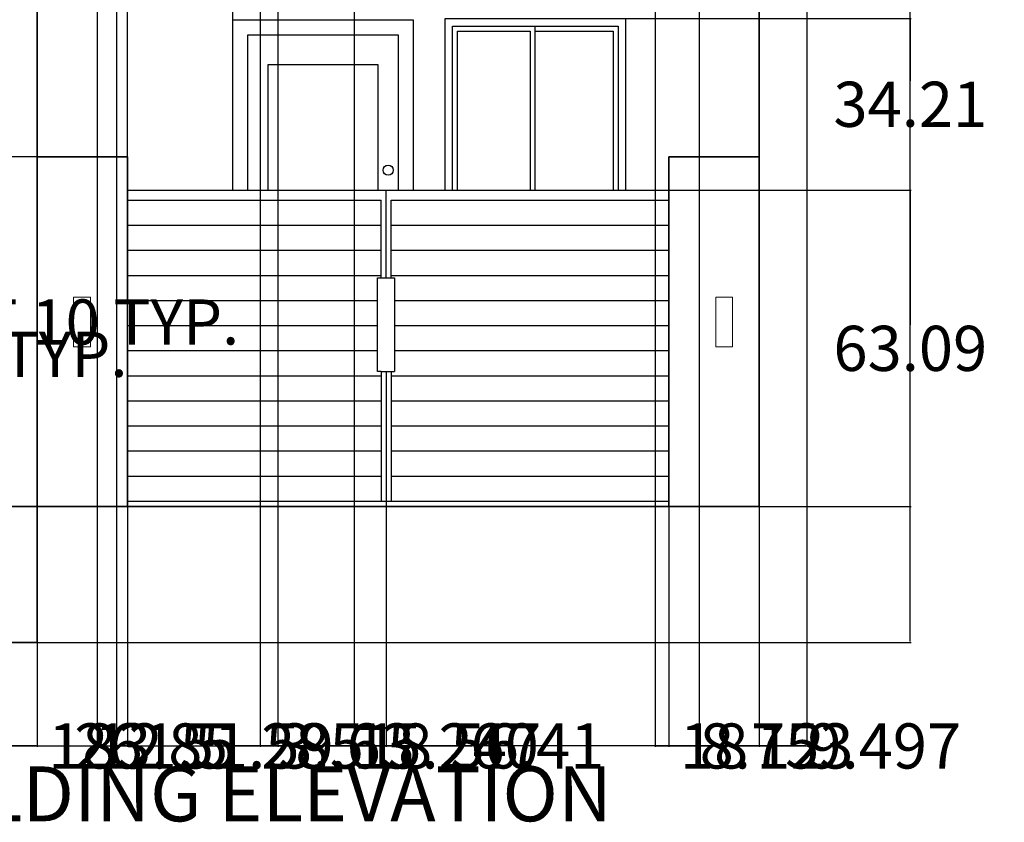
# Model space of a CAD drawing. Units: inches. Extents: x -30 to 323, y -174 to 256.
# Tile 2 of 4: x 127 to 323, y -174 to -14. Entities that reach past the tile are written whole.
import ezdxf

# ---------------------------------------------------------------- set-up
doc = ezdxf.new("R2010")
doc.units = ezdxf.units.IN
doc.header["$MEASUREMENT"] = 0
for name, color, linetype, lineweight in [('A-ANNO-DIMS', 2, 'Continuous', 18), ('A-ANNO-TEXT', 7, 'Continuous', 25), ('A-DOOR', 4, 'Continuous', 25), ('A-ELEV', 7, 'Continuous', 35), ('A-GLAZ', 3, 'Continuous', 25), ('E-LITE', 6, 'Continuous', 18)]:
    doc.layers.add(name, color=color, linetype=linetype, lineweight=lineweight)
doc.styles.get("Standard").update_dxf_attribs({"font": 'arial.ttf'})
doc.dimstyles.get("Standard").update_dxf_attribs({"dimtxt": 9, "dimasz": 0.18, "dimexe": 0.18, "dimexo": 0.0625, "dimgap": 0.09, "dimtad": 0, "dimtih": 1, "dimtoh": 1, "dimdec": 0, "dimzin": 0, "dimdsep": 46, "dimlunit": 3, "dimtxsty": 'Standard', "dimcen": 0.09, "dimadec": 0, "dimazin": 0, "dimtfac": 1, "dimtdec": 0, "dimtofl": 0, "dimtmove": 0, "dimatfit": 3, "dimfxl": 1, "dimtolj": 1, "dimtzin": 0, "dimarcsym": 0})

# ---------------------------------------------------------------- blocks, each defined once
blk = doc.blocks.new('WALL-LIGHT')
blk.add_lwpolyline([(0, 9.92), (3.36, 9.92), (3.36, 0), (0, 0)], close=True)
blk = doc.blocks.new('*D7')
at = {"layer": 'A-ANNO-DIMS', "color": 0, "lineweight": -2, "transparency": 16777216}
for p, q in [((112.24, -69.33), (113.85, -69.33)), ((113.67, -69.15), (113.67, -68.97)), ((112.24, -79.25), (113.85, -79.25)), ((113.67, -79.43), (113.67, -79.61))]:
    blk.add_line(p, q, dxfattribs=at)
at = {"layer": 'A-ANNO-DIMS', "color": 0, "transparency": 16777216}
for points in [[(113.64, -69.15), (113.7, -69.15), (113.67, -69.33)], [(113.64, -79.43), (113.7, -79.43), (113.67, -79.25)]]:
    blk.add_solid(points, dxfattribs=at)
at = {"layer": 'Defpoints', "color": 0, "transparency": 16777216}
for p in [(112.18, -69.33), (113.67, -69.33), (112.18, -79.25)]:
    blk.add_point(p, dxfattribs=at)
at = {"layer": 'A-ANNO-DIMS', "color": 0, "transparency": 16777216, "insert": (113.67, -74.29), "char_height": 9, "attachment_point": 5}
blk.add_mtext('\\A1;WALL LIGHT 10 TYP.', dxfattribs=at)
blk = doc.blocks.new('*D8')
at = {"layer": 'A-ANNO-DIMS', "color": 0, "lineweight": -2, "transparency": 16777216}
for p, q in [((108.82, -79.31), (108.82, -80.91)), ((112.18, -79.31), (112.18, -80.91)), ((109, -80.73), (112, -80.73)), ((112.18, -80.73), (112.36, -80.73))]:
    blk.add_line(p, q, dxfattribs=at)
at = {"layer": 'A-ANNO-DIMS', "color": 0, "transparency": 16777216}
for points in [[(109, -80.7), (109, -80.76), (108.82, -80.73)], [(112, -80.7), (112, -80.76), (112.18, -80.73)]]:
    blk.add_solid(points, dxfattribs=at)
at = {"layer": 'Defpoints', "color": 0, "transparency": 16777216}
for p in [(108.82, -79.25), (112.18, -79.25), (112.18, -80.73)]:
    blk.add_point(p, dxfattribs=at)
at = {"layer": 'A-ANNO-DIMS', "color": 0, "transparency": 16777216, "insert": (130.85, -80.73), "char_height": 9, "attachment_point": 5}
blk.add_mtext('\\A1;3 TYP.', dxfattribs=at)
blk = doc.blocks.new('*D9')
at = {"layer": 'A-ANNO-DIMS', "color": 0, "lineweight": -2, "transparency": 16777216}
for p, q in [((283.63, 8.84), (283.63, -158.98)), ((22.14, -138.22), (22.14, -158.98)), ((22.32, -158.8), (137.5, -158.8)), ((283.45, -158.8), (168.27, -158.8))]:
    blk.add_line(p, q, dxfattribs=at)
at = {"layer": 'A-ANNO-DIMS', "color": 0, "transparency": 16777216}
for points in [[(22.32, -158.77), (22.32, -158.83), (22.14, -158.8)], [(283.45, -158.77), (283.45, -158.83), (283.63, -158.8)]]:
    blk.add_solid(points, dxfattribs=at)
at = {"layer": 'Defpoints', "color": 0, "transparency": 16777216}
for p in [(283.63, 8.91), (22.14, -138.15), (283.63, -158.8)]:
    blk.add_point(p, dxfattribs=at)
at = {"layer": 'A-ANNO-DIMS', "color": 0, "transparency": 16777216, "insert": (152.88, -158.8), "char_height": 9, "attachment_point": 5}
blk.add_mtext('\\A1;261.5', dxfattribs=at)
blk = doc.blocks.new('*D10')
at = {"layer": 'A-ANNO-DIMS', "color": 0, "lineweight": -2, "transparency": 16777216}
for p, q in [((15.03, 229.9), (304.46, 229.9)), ((304.28, 229.72), (304.28, 50.56)), ((304.28, -137.97), (304.28, 41.18)), ((22.2, -138.15), (304.46, -138.15))]:
    blk.add_line(p, q, dxfattribs=at)
at = {"layer": 'A-ANNO-DIMS', "color": 0, "transparency": 16777216}
for points in [[(304.25, 229.72), (304.31, 229.72), (304.28, 229.9)], [(304.25, -137.97), (304.31, -137.97), (304.28, -138.15)]]:
    blk.add_solid(points, dxfattribs=at)
at = {"layer": 'Defpoints', "color": 0, "transparency": 16777216}
for p in [(14.97, 229.9), (22.14, -138.15), (304.28, -138.15)]:
    blk.add_point(p, dxfattribs=at)
at = {"layer": 'A-ANNO-DIMS', "color": 0, "transparency": 16777216, "insert": (304.28, 45.87), "char_height": 9, "attachment_point": 5}
blk.add_mtext('\\A1;368.05', dxfattribs=at)
blk = doc.blocks.new('*D22')
at = {"layer": 'A-ANNO-DIMS', "color": 0, "lineweight": -2, "transparency": 16777216}
for p, q in [((92.12, -60.62), (92.12, 250.73)), ((92.3, 250.55), (95.9, 250.55)), ((129.96, 250.55), (126.35, 250.55)), ((130.14, -111.03), (130.14, 250.73))]:
    blk.add_line(p, q, dxfattribs=at)
at = {"layer": 'A-ANNO-DIMS', "color": 0, "transparency": 16777216}
for points in [[(92.3, 250.58), (92.3, 250.52), (92.12, 250.55)], [(129.96, 250.58), (129.96, 250.52), (130.14, 250.55)]]:
    blk.add_solid(points, dxfattribs=at)
at = {"layer": 'Defpoints', "color": 0, "transparency": 16777216}
for p in [(130.14, 250.55), (92.12, -60.68), (130.14, -111.09)]:
    blk.add_point(p, dxfattribs=at)
at = {"layer": 'A-ANNO-DIMS', "color": 0, "transparency": 16777216, "insert": (111.13, 250.55), "char_height": 9, "attachment_point": 5}
blk.add_mtext('\\A1;38.02', dxfattribs=at)
blk = doc.blocks.new('*D23')
at = {"layer": 'A-ANNO-DIMS', "color": 0, "lineweight": -2, "transparency": 16777216}
for p, q in [((22.14, -138.22), (22.14, -158.98)), ((130.14, -138.22), (130.14, -158.98)), ((22.32, -158.8), (66.52, -158.8)), ((129.96, -158.8), (85.75, -158.8))]:
    blk.add_line(p, q, dxfattribs=at)
at = {"layer": 'A-ANNO-DIMS', "color": 0, "transparency": 16777216}
for points in [[(22.32, -158.77), (22.32, -158.83), (22.14, -158.8)], [(129.96, -158.77), (129.96, -158.83), (130.14, -158.8)]]:
    blk.add_solid(points, dxfattribs=at)
at = {"layer": 'Defpoints', "color": 0, "transparency": 16777216}
for p in [(22.14, -138.15), (130.14, -138.15), (130.14, -158.8)]:
    blk.add_point(p, dxfattribs=at)
at = {"layer": 'A-ANNO-DIMS', "color": 0, "transparency": 16777216, "insert": (76.14, -158.8), "char_height": 9, "attachment_point": 5}
blk.add_mtext('\\A1;108', dxfattribs=at)
blk = doc.blocks.new('*D44')
at = {"layer": 'A-ANNO-DIMS', "color": 0, "lineweight": -2, "transparency": 16777216}
for p, q in [((142.14, 20.84), (142.14, -158.98)), ((130.14, 8.84), (130.14, -158.98)), ((130.32, -158.8), (141.96, -158.8)), ((142.14, -158.8), (142.32, -158.8))]:
    blk.add_line(p, q, dxfattribs=at)
at = {"layer": 'A-ANNO-DIMS', "color": 0, "transparency": 16777216}
for points in [[(130.32, -158.77), (130.32, -158.83), (130.14, -158.8)], [(141.96, -158.77), (141.96, -158.83), (142.14, -158.8)]]:
    blk.add_solid(points, dxfattribs=at)
at = {"layer": 'Defpoints', "color": 0, "transparency": 16777216}
for p in [(142.14, 20.91), (130.14, 8.91), (142.14, -158.8)]:
    blk.add_point(p, dxfattribs=at)
at = {"layer": 'A-ANNO-DIMS', "color": 0, "transparency": 16777216, "insert": (148.38, -158.8), "char_height": 9, "attachment_point": 5}
blk.add_mtext('\\A1;12', dxfattribs=at)
blk = doc.blocks.new('*D45')
at = {"layer": 'A-ANNO-DIMS', "color": 0, "lineweight": -2, "transparency": 16777216}
for p, q in [((145.99, 36.26), (145.99, -158.98)), ((142.14, 20.84), (142.14, -158.98)), ((142.32, -158.8), (145.81, -158.8)), ((145.99, -158.8), (146.17, -158.8))]:
    blk.add_line(p, q, dxfattribs=at)
at = {"layer": 'A-ANNO-DIMS', "color": 0, "transparency": 16777216}
for points in [[(142.32, -158.77), (142.32, -158.83), (142.14, -158.8)], [(145.81, -158.77), (145.81, -158.83), (145.99, -158.8)]]:
    blk.add_solid(points, dxfattribs=at)
at = {"layer": 'Defpoints', "color": 0, "transparency": 16777216}
for p in [(145.99, 36.33), (142.14, 20.91), (145.99, -158.8)]:
    blk.add_point(p, dxfattribs=at)
at = {"layer": 'A-ANNO-DIMS', "color": 0, "transparency": 16777216, "insert": (157.98, -158.8), "char_height": 9, "attachment_point": 5}
blk.add_mtext('\\A1;3.85', dxfattribs=at)
blk = doc.blocks.new('*D46')
at = {"layer": 'A-ANNO-DIMS', "color": 0, "lineweight": -2, "transparency": 16777216}
for p, q in [((145.99, 36.26), (145.99, -158.98)), ((174.62, 36.26), (174.62, -158.98)), ((146.17, -158.8), (174.44, -158.8)), ((174.62, -158.8), (174.8, -158.8))]:
    blk.add_line(p, q, dxfattribs=at)
at = {"layer": 'A-ANNO-DIMS', "color": 0, "transparency": 16777216}
for points in [[(146.17, -158.77), (146.17, -158.83), (145.99, -158.8)], [(174.44, -158.77), (174.44, -158.83), (174.62, -158.8)]]:
    blk.add_solid(points, dxfattribs=at)
at = {"layer": 'Defpoints', "color": 0, "transparency": 16777216}
for p in [(145.99, 36.33), (174.62, 36.33), (174.62, -158.8)]:
    blk.add_point(p, dxfattribs=at)
at = {"layer": 'A-ANNO-DIMS', "color": 0, "transparency": 16777216, "insert": (190.15, -158.8), "char_height": 9, "attachment_point": 5}
blk.add_mtext('\\A1;28.63', dxfattribs=at)
blk = doc.blocks.new('*D47')
at = {"layer": 'A-ANNO-DIMS', "color": 0, "lineweight": -2, "transparency": 16777216}
for p, q in [((174.62, 36.26), (174.62, -158.98)), ((178.14, 32.84), (178.14, -158.98)), ((174.8, -158.8), (177.96, -158.8)), ((178.14, -158.8), (178.32, -158.8))]:
    blk.add_line(p, q, dxfattribs=at)
at = {"layer": 'A-ANNO-DIMS', "color": 0, "transparency": 16777216}
for points in [[(174.8, -158.77), (174.8, -158.83), (174.62, -158.8)], [(177.96, -158.77), (177.96, -158.83), (178.14, -158.8)]]:
    blk.add_solid(points, dxfattribs=at)
at = {"layer": 'Defpoints', "color": 0, "transparency": 16777216}
for p in [(174.62, 36.33), (178.14, 32.91), (178.14, -158.8)]:
    blk.add_point(p, dxfattribs=at)
at = {"layer": 'A-ANNO-DIMS', "color": 0, "transparency": 16777216, "insert": (193.6, -158.8), "char_height": 9, "attachment_point": 5}
blk.add_mtext('\\A1;3.518', dxfattribs=at)
blk = doc.blocks.new('*D48')
at = {"layer": 'A-ANNO-DIMS', "color": 0, "lineweight": -2, "transparency": 16777216}
for p, q in [((178.14, 32.84), (178.14, -158.98)), ((193.38, 32.84), (193.38, -158.98)), ((178.32, -158.8), (193.2, -158.8)), ((193.38, -158.8), (193.56, -158.8))]:
    blk.add_line(p, q, dxfattribs=at)
at = {"layer": 'A-ANNO-DIMS', "color": 0, "transparency": 16777216}
for points in [[(178.32, -158.77), (178.32, -158.83), (178.14, -158.8)], [(193.2, -158.77), (193.2, -158.83), (193.38, -158.8)]]:
    blk.add_solid(points, dxfattribs=at)
at = {"layer": 'Defpoints', "color": 0, "transparency": 16777216}
for p in [(178.14, 32.91), (193.38, 32.91), (193.38, -158.8)]:
    blk.add_point(p, dxfattribs=at)
at = {"layer": 'A-ANNO-DIMS', "color": 0, "transparency": 16777216, "insert": (211.91, -158.8), "char_height": 9, "attachment_point": 5}
blk.add_mtext('\\A1;15.247', dxfattribs=at)
blk = doc.blocks.new('*D49')
at = {"layer": 'A-ANNO-DIMS', "color": 0, "lineweight": -2, "transparency": 16777216}
for p, q in [((193.38, 32.84), (193.38, -158.98)), ((253.38, 32.84), (253.38, -158.98)), ((193.56, -158.8), (216.84, -158.8)), ((253.2, -158.8), (229.93, -158.8))]:
    blk.add_line(p, q, dxfattribs=at)
at = {"layer": 'A-ANNO-DIMS', "color": 0, "transparency": 16777216}
for points in [[(193.56, -158.77), (193.56, -158.83), (193.38, -158.8)], [(253.2, -158.77), (253.2, -158.83), (253.38, -158.8)]]:
    blk.add_solid(points, dxfattribs=at)
at = {"layer": 'Defpoints', "color": 0, "transparency": 16777216}
for p in [(193.38, 32.91), (253.38, 32.91), (253.38, -158.8)]:
    blk.add_point(p, dxfattribs=at)
at = {"layer": 'A-ANNO-DIMS', "color": 0, "transparency": 16777216, "insert": (223.38, -158.8), "char_height": 9, "attachment_point": 5}
blk.add_mtext('\\A1;60', dxfattribs=at)
blk = doc.blocks.new('*D50')
at = {"layer": 'A-ANNO-DIMS', "color": 0, "lineweight": -2, "transparency": 16777216}
for p, q in [((253.38, 32.84), (253.38, -158.98)), ((262.14, 32.84), (262.14, -158.98)), ((253.56, -158.8), (261.96, -158.8)), ((262.14, -158.8), (262.32, -158.8))]:
    blk.add_line(p, q, dxfattribs=at)
at = {"layer": 'A-ANNO-DIMS', "color": 0, "transparency": 16777216}
for points in [[(253.56, -158.77), (253.56, -158.83), (253.38, -158.8)], [(261.96, -158.77), (261.96, -158.83), (262.14, -158.8)]]:
    blk.add_solid(points, dxfattribs=at)
at = {"layer": 'Defpoints', "color": 0, "transparency": 16777216}
for p in [(253.38, 32.91), (262.14, 32.91), (262.14, -158.8)]:
    blk.add_point(p, dxfattribs=at)
at = {"layer": 'A-ANNO-DIMS', "color": 0, "transparency": 16777216, "insert": (277.6, -158.8), "char_height": 9, "attachment_point": 5}
blk.add_mtext('\\A1;8.753', dxfattribs=at)
blk = doc.blocks.new('*D51')
at = {"layer": 'A-ANNO-DIMS', "color": 0, "lineweight": -2, "transparency": 16777216}
for p, q in [((262.14, 32.84), (262.14, -158.98)), ((274.14, 20.84), (274.14, -158.98)), ((262.32, -158.8), (273.96, -158.8)), ((274.14, -158.8), (274.32, -158.8))]:
    blk.add_line(p, q, dxfattribs=at)
at = {"layer": 'A-ANNO-DIMS', "color": 0, "transparency": 16777216}
for points in [[(262.32, -158.77), (262.32, -158.83), (262.14, -158.8)], [(273.96, -158.77), (273.96, -158.83), (274.14, -158.8)]]:
    blk.add_solid(points, dxfattribs=at)
at = {"layer": 'Defpoints', "color": 0, "transparency": 16777216}
for p in [(262.14, 32.91), (274.14, 20.91), (274.14, -158.8)]:
    blk.add_point(p, dxfattribs=at)
at = {"layer": 'A-ANNO-DIMS', "color": 0, "transparency": 16777216, "insert": (280.38, -158.8), "char_height": 9, "attachment_point": 5}
blk.add_mtext('\\A1;12', dxfattribs=at)
blk = doc.blocks.new('*D52')
at = {"layer": 'A-ANNO-DIMS', "color": 0, "lineweight": -2, "transparency": 16777216}
for p, q in [((148.14, -47.95), (148.14, 250.73)), ((148.32, 250.55), (168.97, 250.55)), ((169.15, -13.98), (169.15, 250.73)), ((169.15, 250.55), (169.33, 250.55))]:
    blk.add_line(p, q, dxfattribs=at)
at = {"layer": 'A-ANNO-DIMS', "color": 0, "transparency": 16777216}
for points in [[(148.32, 250.58), (148.32, 250.52), (148.14, 250.55)], [(168.97, 250.58), (168.97, 250.52), (169.15, 250.55)]]:
    blk.add_solid(points, dxfattribs=at)
at = {"layer": 'Defpoints', "color": 0, "transparency": 16777216}
for p in [(169.15, 250.55), (169.15, -14.04), (148.14, -48.01)]:
    blk.add_point(p, dxfattribs=at)
at = {"layer": 'A-ANNO-DIMS', "color": 0, "transparency": 16777216, "insert": (188.16, 250.55), "char_height": 9, "attachment_point": 5}
blk.add_mtext('\\A1;21.014', dxfattribs=at)
blk = doc.blocks.new('*D56')
at = {"layer": 'A-ANNO-DIMS', "color": 0, "lineweight": -2, "transparency": 16777216}
for p, q in [((130.14, -111.16), (130.14, -158.98)), ((148.14, -111.16), (148.14, -158.98)), ((130.32, -158.8), (133.01, -158.8)), ((147.96, -158.8), (145.26, -158.8))]:
    blk.add_line(p, q, dxfattribs=at)
at = {"layer": 'A-ANNO-DIMS', "color": 0, "transparency": 16777216}
for points in [[(130.32, -158.77), (130.32, -158.83), (130.14, -158.8)], [(147.96, -158.77), (147.96, -158.83), (148.14, -158.8)]]:
    blk.add_solid(points, dxfattribs=at)
at = {"layer": 'Defpoints', "color": 0, "transparency": 16777216}
for p in [(130.14, -111.09), (148.14, -111.09), (148.14, -158.8)]:
    blk.add_point(p, dxfattribs=at)
at = {"layer": 'A-ANNO-DIMS', "color": 0, "transparency": 16777216, "insert": (139.14, -158.8), "char_height": 9, "attachment_point": 5}
blk.add_mtext('\\A1;18', dxfattribs=at)
blk = doc.blocks.new('*D57')
at = {"layer": 'A-ANNO-DIMS', "color": 0, "lineweight": -2, "transparency": 16777216}
for p, q in [((148.14, -111.16), (148.14, -158.98)), ((199.73, -111.16), (199.73, -158.98)), ((148.32, -158.8), (158.65, -158.8)), ((199.55, -158.8), (189.22, -158.8))]:
    blk.add_line(p, q, dxfattribs=at)
at = {"layer": 'A-ANNO-DIMS', "color": 0, "transparency": 16777216}
for points in [[(148.32, -158.77), (148.32, -158.83), (148.14, -158.8)], [(199.55, -158.77), (199.55, -158.83), (199.73, -158.8)]]:
    blk.add_solid(points, dxfattribs=at)
at = {"layer": 'Defpoints', "color": 0, "transparency": 16777216}
for p in [(148.14, -111.09), (199.73, -111.09), (199.73, -158.8)]:
    blk.add_point(p, dxfattribs=at)
at = {"layer": 'A-ANNO-DIMS', "color": 0, "transparency": 16777216, "insert": (173.93, -158.8), "char_height": 9, "attachment_point": 5}
blk.add_mtext('\\A1;51.59', dxfattribs=at)
blk = doc.blocks.new('*D58')
at = {"layer": 'A-ANNO-DIMS', "color": 0, "lineweight": -2, "transparency": 16777216}
for p, q in [((199.73, -111.16), (199.73, -158.98)), ((256.14, -111.16), (256.14, -158.98)), ((199.91, -158.8), (213.53, -158.8)), ((255.96, -158.8), (242.34, -158.8))]:
    blk.add_line(p, q, dxfattribs=at)
at = {"layer": 'A-ANNO-DIMS', "color": 0, "transparency": 16777216}
for points in [[(199.91, -158.77), (199.91, -158.83), (199.73, -158.8)], [(255.96, -158.77), (255.96, -158.83), (256.14, -158.8)]]:
    blk.add_solid(points, dxfattribs=at)
at = {"layer": 'Defpoints', "color": 0, "transparency": 16777216}
for p in [(199.73, -111.09), (256.14, -111.09), (256.14, -158.8)]:
    blk.add_point(p, dxfattribs=at)
at = {"layer": 'A-ANNO-DIMS', "color": 0, "transparency": 16777216, "insert": (227.93, -158.8), "char_height": 9, "attachment_point": 5}
blk.add_mtext('\\A1;56.41', dxfattribs=at)
blk = doc.blocks.new('*D59')
at = {"layer": 'A-ANNO-DIMS', "color": 0, "lineweight": -2, "transparency": 16777216}
for p, q in [((256.14, -111.16), (256.14, -158.98)), ((274.14, -111.16), (274.14, -158.98)), ((256.32, -158.8), (259.01, -158.8)), ((273.96, -158.8), (271.26, -158.8))]:
    blk.add_line(p, q, dxfattribs=at)
at = {"layer": 'A-ANNO-DIMS', "color": 0, "transparency": 16777216}
for points in [[(256.32, -158.77), (256.32, -158.83), (256.14, -158.8)], [(273.96, -158.77), (273.96, -158.83), (274.14, -158.8)]]:
    blk.add_solid(points, dxfattribs=at)
at = {"layer": 'Defpoints', "color": 0, "transparency": 16777216}
for p in [(256.14, -111.09), (274.14, -111.09), (274.14, -158.8)]:
    blk.add_point(p, dxfattribs=at)
at = {"layer": 'A-ANNO-DIMS', "color": 0, "transparency": 16777216, "insert": (265.14, -158.8), "char_height": 9, "attachment_point": 5}
blk.add_mtext('\\A1;18', dxfattribs=at)
blk = doc.blocks.new('*D60')
at = {"layer": 'A-ANNO-DIMS', "color": 0, "lineweight": -2, "transparency": 16777216}
for p, q in [((283.63, 8.84), (283.63, -158.98)), ((274.14, -111.16), (274.14, -158.98)), ((274.32, -158.8), (283.45, -158.8)), ((283.63, -158.8), (283.81, -158.8))]:
    blk.add_line(p, q, dxfattribs=at)
at = {"layer": 'A-ANNO-DIMS', "color": 0, "transparency": 16777216}
for points in [[(274.32, -158.77), (274.32, -158.83), (274.14, -158.8)], [(283.45, -158.77), (283.45, -158.83), (283.63, -158.8)]]:
    blk.add_solid(points, dxfattribs=at)
at = {"layer": 'Defpoints', "color": 0, "transparency": 16777216}
for p in [(283.63, 8.91), (274.14, -111.09), (283.63, -158.8)]:
    blk.add_point(p, dxfattribs=at)
at = {"layer": 'A-ANNO-DIMS', "color": 0, "transparency": 16777216, "insert": (299.09, -158.8), "char_height": 9, "attachment_point": 5}
blk.add_mtext('\\A1;9.497', dxfattribs=at)
blk = doc.blocks.new('*D61')
at = {"layer": 'A-ANNO-DIMS', "color": 0, "lineweight": -2, "transparency": 16777216}
for p, q in [((148.07, -41.35), (-5.86, -41.35)), ((-5.68, -41.53), (-5.68, -71.54)), ((-5.68, -110.91), (-5.68, -80.91)), ((130.07, -111.09), (-5.86, -111.09))]:
    blk.add_line(p, q, dxfattribs=at)
at = {"layer": 'A-ANNO-DIMS', "color": 0, "transparency": 16777216}
for points in [[(-5.71, -41.53), (-5.65, -41.53), (-5.68, -41.35)], [(-5.71, -110.91), (-5.65, -110.91), (-5.68, -111.09)]]:
    blk.add_solid(points, dxfattribs=at)
at = {"layer": 'Defpoints', "color": 0, "transparency": 16777216}
for p in [(-5.68, -41.35), (148.14, -41.35), (130.14, -111.09)]:
    blk.add_point(p, dxfattribs=at)
at = {"layer": 'A-ANNO-DIMS', "color": 0, "transparency": 16777216, "insert": (-5.68, -76.22), "char_height": 9, "attachment_point": 5}
blk.add_mtext('\\A1;69.74', dxfattribs=at)
blk = doc.blocks.new('*D62')
at = {"layer": 'A-ANNO-DIMS', "color": 0, "lineweight": -2, "transparency": 16777216}
for p, q in [((256.2, -48.01), (304.46, -48.01)), ((304.28, -48.19), (304.28, -74.86)), ((304.28, -110.91), (304.28, -84.24)), ((274.2, -111.09), (304.46, -111.09))]:
    blk.add_line(p, q, dxfattribs=at)
at = {"layer": 'A-ANNO-DIMS', "color": 0, "transparency": 16777216}
for points in [[(304.25, -48.19), (304.31, -48.19), (304.28, -48.01)], [(304.25, -110.91), (304.31, -110.91), (304.28, -111.09)]]:
    blk.add_solid(points, dxfattribs=at)
at = {"layer": 'Defpoints', "color": 0, "transparency": 16777216}
for p in [(256.14, -48.01), (304.28, -48.01), (274.14, -111.09)]:
    blk.add_point(p, dxfattribs=at)
at = {"layer": 'A-ANNO-DIMS', "color": 0, "transparency": 16777216, "insert": (304.28, -79.55), "char_height": 9, "attachment_point": 5}
blk.add_mtext('\\A1;63.09', dxfattribs=at)
blk = doc.blocks.new('*D63')
at = {"layer": 'A-ANNO-DIMS', "color": 0, "lineweight": -2, "transparency": 16777216}
for p, q in [((247.55, -13.8), (304.46, -13.8)), ((304.28, -13.98), (304.28, -26.22)), ((304.28, -47.83), (304.28, -35.59)), ((256.2, -48.01), (304.46, -48.01))]:
    blk.add_line(p, q, dxfattribs=at)
at = {"layer": 'A-ANNO-DIMS', "color": 0, "transparency": 16777216}
for points in [[(304.25, -13.98), (304.31, -13.98), (304.28, -13.8)], [(304.25, -47.83), (304.31, -47.83), (304.28, -48.01)]]:
    blk.add_solid(points, dxfattribs=at)
at = {"layer": 'Defpoints', "color": 0, "transparency": 16777216}
for p in [(247.49, -13.8), (304.28, -13.8), (256.14, -48.01)]:
    blk.add_point(p, dxfattribs=at)
at = {"layer": 'A-ANNO-DIMS', "color": 0, "transparency": 16777216, "insert": (304.28, -30.9), "char_height": 9, "attachment_point": 5}
blk.add_mtext('\\A1;34.21', dxfattribs=at)

msp = doc.modelspace()

# ---------------------------------------------------------------- linework, layer by layer
at = {"layer": 'A-DOOR'}
for p, q in [((148.136, -48.0084), (256.136, -48.0084)), ((199.728, -65.4893), (199.728, -48.0084)), ((148.136, -50), (198.728, -50)), ((198.728, -65.4893), (198.728, -50)), ((200.728, -65.4893), (200.728, -50)), ((200.728, -65.4893), (200.728, -50)), ((200.728, -50), (256.136, -50)), ((148.136, -55), (198.728, -55)), ((200.728, -55), (256.136, -55)), ((148.136, -60), (198.728, -60)), ((200.728, -60), (256.136, -60)), ((148.136, -65), (198.728, -65)), ((198.728, -65.4893), (200.728, -65.4893)), ((200.728, -65), (256.136, -65)), ((148.136, -70), (198.0459, -70)), ((201.4101, -70), (256.136, -70)), ((148.136, -75), (198.0459, -75)), ((201.4101, -75), (256.136, -75)), ((148.136, -80), (198.0459, -80)), ((201.4101, -80), (256.136, -80)), ((198.728, -84.1897), (198.728, -110)), ((198.728, -84.1897), (201.4101, -84.1897)), ((199.728, -84.1897), (199.728, -111.0941)), ((200.728, -84.1897), (200.728, -110)), ((148.136, -85), (198.728, -85)), ((200.728, -85), (256.136, -85)), ((148.136, -90), (198.728, -90)), ((200.728, -90), (256.136, -90)), ((148.136, -95), (198.728, -95)), ((200.728, -95), (256.136, -95)), ((148.136, -100), (198.728, -100)), ((200.728, -100), (256.136, -100)), ((148.136, -105), (198.728, -105)), ((200.728, -105), (256.136, -105)), ((148.136, -110), (256.136, -110))]:
    msp.add_line(p, q, dxfattribs=at)
for points in [[(169.1503, -48.0084), (169.1503, -14.04), (205.1503, -14.04), (205.1503, -48.0084)], [(172.1503, -48.0084), (172.1503, -17.063), (202.1503, -17.063), (202.1503, -48.0084)], [(198.1503, -48.0084), (198.1503, -23.063), (176.1503, -23.063), (176.1503, -48.0084)], [(198.728, -84.1897), (198.0459, -84.1897), (198.0459, -65.4893), (198.728, -65.4893)], [(200.728, -65.4893), (201.4101, -65.4893), (201.4101, -84.1897)]]:
    msp.add_lwpolyline(points, dxfattribs=at)
msp.add_circle((200.1503, -44.04), 1, dxfattribs=at)
at = {"layer": 'A-ELEV'}
msp.add_lwpolyline([(130.136, 149.9059), (274.136, 149.9059), (274.136, 128.9059), (279.5695, 128.9059), (279.5695, 104.9059), (274.136, 104.9059), (274.136, 20.9059), (283.6325, 20.9059), (283.6325, 8.9059), (274.136, 8.9059), (274.136, -111.0941), (22.136, -111.0941), (22.136, 224.9059), (130.136, 224.9059), (130.136, -111.0941)], dxfattribs=at)
for points in [[(130.136, -41.3495), (148.136, -41.3495), (148.136, -111.0941), (130.136, -111.0941)], [(256.136, -41.3495), (274.136, -41.3495), (274.136, -111.0941), (256.136, -111.0941)], [(92.2427, -111.0941), (130.136, -111.0941), (130.136, -138.1526), (92.2427, -138.1526)]]:
    msp.add_lwpolyline(points, close=True, dxfattribs=at)
at = {"layer": 'A-GLAZ'}
msp.add_line((229.4887, -48.0084), (229.4887, -15.301), dxfattribs=at)
for points in [[(211.4887, -48.0084), (211.4887, -13.801), (247.4887, -13.801), (247.4887, -48.0084)], [(212.9887, -48.0084), (212.9887, -15.301), (229.4887, -15.301), (245.9887, -15.301), (245.9887, -48.0084)], [(213.9887, -48.0084), (213.9887, -16.301), (228.4887, -16.301)], [(228.4887, -16.3009), (228.4887, -48.0084)], [(229.4887, -16.301), (244.9887, -16.301), (244.9887, -48.0084)]]:
    msp.add_lwpolyline(points, dxfattribs=at)

# ---------------------------------------------------------------- block references
at = {"layer": 'E-LITE'}
for p in [(137.411, -79.246), (265.4672, -79.246)]:
    msp.add_blockref('WALL-LIGHT', p, dxfattribs=at)

# ---------------------------------------------------------------- texts
at = {"layer": 'A-ANNO-TEXT'}
msp.add_text('G+1 BUILDING ELEVATION', height=10.938735, dxfattribs=at).set_placement((64.0004, -173.8227))

# ---------------------------------------------------------------- dimensions: what is measured, and where the dimension line sits
at = {"layer": 'A-ANNO-DIMS'}
for base, p1, p2, override, picture, middle in [((130.136, 250.5457), (92.1189, -60.6838), (130.136, -111.0941), {"dimdec": 2, "dimlfac": 1, "dimrnd": 0, "dimzin": 0, "dimdsep": 46, "dimlunit": 2}, '*D22', (111.1274, 250.5457)), ((169.1503, 250.5457), (148.136, -48.0084), (169.1503, -14.04), {"dimdec": 3, "dimlfac": 1, "dimrnd": 0, "dimzin": 0, "dimdsep": 46, "dimlunit": 2}, '*D52', (188.1601, 250.5457)), ((145.9862, -158.8026), (142.136, 20.9059), (145.9862, 36.3257), {"dimdec": 2, "dimlfac": 1, "dimrnd": 0, "dimzin": 0, "dimdsep": 46, "dimlunit": 2}, '*D45', (157.9758, -158.8026)), ((174.6182, -158.8026), (145.9862, 36.3257), (174.6182, 36.3257), {"dimdec": 2, "dimlfac": 1, "dimrnd": 0, "dimzin": 0, "dimdsep": 46, "dimlunit": 2}, '*D46', (190.1501, -158.8026)), ((178.136, -158.8026), (174.6182, 36.3257), (178.136, 32.9059), {"dimdec": 3, "dimlfac": 1, "dimrnd": 0, "dimzin": 0, "dimdsep": 46, "dimlunit": 2}, '*D47', (193.5973, -158.8026)), ((193.3831, -158.8026), (178.136, 32.9059), (193.3831, 32.9059), {"dimdec": 3, "dimlfac": 1, "dimrnd": 0, "dimzin": 0, "dimdsep": 46, "dimlunit": 2}, '*D48', (211.9109, -158.8026)), ((253.3831, -158.8026), (193.3831, 32.9059), (253.3831, 32.9059), {"dimdec": 0, "dimlfac": 1, "dimrnd": 0, "dimzin": 0, "dimdsep": 46, "dimlunit": 2}, '*D49', (223.3831, -158.8026)), ((262.136, -158.8026), (253.3831, 32.9059), (262.136, 32.9059), {"dimdec": 3, "dimlfac": 1, "dimrnd": 0, "dimzin": 0, "dimdsep": 46, "dimlunit": 2}, '*D50', (277.5973, -158.8026)), ((274.136, -158.8026), (262.136, 32.9059), (274.136, 20.9059), {"dimdec": 0, "dimlfac": 1, "dimrnd": 0, "dimzin": 0, "dimdsep": 46, "dimlunit": 2}, '*D51', (280.3824, -158.8026)), ((142.136, -158.8026), (130.136, 8.9059), (142.136, 20.9059), {"dimdec": 0, "dimlfac": 1, "dimrnd": 0, "dimzin": 0, "dimdsep": 46, "dimlunit": 2}, '*D44', (148.3824, -158.8026)), ((283.6325, -158.8026), (22.136, -138.1526), (283.6325, 8.9059), {"dimdec": 1, "dimlfac": 1, "dimrnd": 0, "dimzin": 0, "dimdsep": 46, "dimlunit": 2}, '*D9', (152.8843, -158.8026)), ((283.63254, -158.80263), (274.13598, -111.09408), (283.63254, 8.90592), {"dimdec": 3, "dimlfac": 1, "dimrnd": 0, "dimzin": 0, "dimdsep": 46, "dimlunit": 2}, '*D60', (299.08774, -158.80263)), ((148.136, -158.8026), (130.136, -111.0941), (148.136, -111.0941), {"dimdec": 0, "dimlfac": 1, "dimrnd": 0, "dimzin": 0, "dimdsep": 46, "dimlunit": 2}, '*D56', (139.136, -158.8026)), ((199.728, -158.8026), (148.136, -111.0941), (199.728, -111.0941), {"dimdec": 2, "dimlfac": 1, "dimrnd": 0, "dimzin": 0, "dimdsep": 46, "dimlunit": 2}, '*D57', (173.932, -158.8026)), ((256.136, -158.8026), (199.728, -111.0941), (256.136, -111.0941), {"dimdec": 2, "dimlfac": 1, "dimrnd": 0, "dimzin": 0, "dimdsep": 46, "dimlunit": 2}, '*D58', (227.932, -158.8026)), ((274.136, -158.8026), (256.136, -111.0941), (274.136, -111.0941), {"dimdec": 0, "dimlfac": 1, "dimrnd": 0, "dimzin": 0, "dimdsep": 46, "dimlunit": 2}, '*D59', (265.136, -158.8026)), ((130.136, -158.8026), (22.136, -138.1526), (130.136, -138.1526), {"dimdec": 0, "dimlfac": 1, "dimrnd": 0, "dimzin": 0, "dimdsep": 46, "dimlunit": 2}, '*D23', (76.136, -158.8026))]:
    dim = msp.add_linear_dim(base=base, p1=p1, p2=p2, dimstyle='Standard', override=override, dxfattribs=at)
    dim.commit()
    dim.dimension.update_dxf_attribs({"geometry": picture, "text_midpoint": middle})
for base, p1, p2, picture, middle in [((304.2825, -138.1526), (14.9689, 229.8957), (22.136, -138.1526), '*D10', (304.2825, 45.8715)), ((304.2825, -13.801), (256.136, -48.0084), (247.4887, -13.801), '*D63', (304.2825, -30.9047)), ((-5.6811, -41.3495), (130.136, -111.0941), (148.136, -41.3495), '*D61', (-5.6811, -76.2218)), ((304.2825, -48.0084), (274.136, -111.0941), (256.136, -48.0084), '*D62', (304.2825, -79.5512))]:
    dim = msp.add_linear_dim(base=base, p1=p1, p2=p2, angle=90, dimstyle='Standard', override={"dimdec": 2, "dimlfac": 1, "dimrnd": 0, "dimzin": 0, "dimdsep": 46, "dimlunit": 2}, dxfattribs=at)
    dim.commit()
    dim.dimension.update_dxf_attribs({"geometry": picture, "text_midpoint": middle})
dim = msp.add_linear_dim(base=(113.6666, -69.3307), p1=(112.1793, -79.2457), p2=(112.1793, -69.3307), angle=90, text='WALL LIGHT <> TYP.', dimstyle='Standard', override={"dimdec": 0, "dimlfac": 1, "dimrnd": 0, "dimzin": 0, "dimdsep": 46, "dimlunit": 2}, dxfattribs=at)
dim.commit()
dim.dimension.update_dxf_attribs({"geometry": '*D7', "text_midpoint": (113.6666, -74.2882)})
dim = msp.add_linear_dim(base=(112.1793, -80.7329), p1=(108.8152, -79.2457), p2=(112.1793, -79.2457), text='<> TYP.', dimstyle='Standard', override={"dimdec": 0, "dimlfac": 1, "dimrnd": 0, "dimzin": 0, "dimdsep": 46, "dimlunit": 2}, dxfattribs=at)
dim.commit()
dim.dimension.update_dxf_attribs({"geometry": '*D8', "text_midpoint": (130.8545, -80.7329)})

doc.saveas('drawing.dxf')
